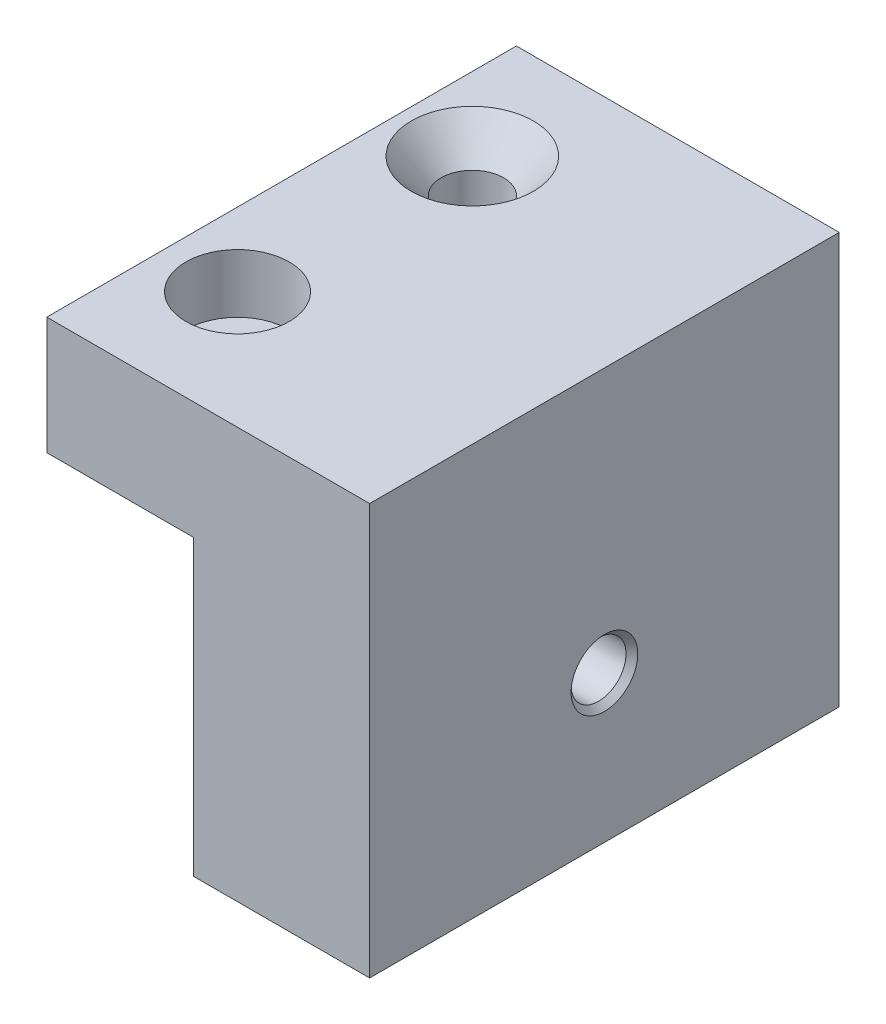
SolidWorks part; units mm, degrees
material "Plain Carbon Steel"
ref_plane "Front Plane" through (0, 0, 0) normal (0, 0, 1) x (1, 0, 0)
ref_plane "Top Plane" through (0, 0, 0) normal (0, 1, 0) x (1, 0, 0)
ref_plane "Right Plane" through (0, 0, 0) normal (1, 0, 0) x (0, 0, -1)
sketch "Block Profile Sketch" plane through (0, 0, 0) normal (0, 0, 1) x (1, 0, 0)
  line L2 (0, 12.7) -> (19.05, 12.7)
  line L3 (0, 0) -> (0, -31.75)
  line L4 (0, -31.75) -> (19.05, -31.75)
  line L5 (19.05, 12.7) -> (19.05, -31.75)
  line L6 (0, 0) -> (-15.875, 0)
  line L8 (0, 12.7) -> (-15.875, 12.7)
  line L9 (-15.875, 0) -> (-15.875, 12.7)
  dimension "D1" = 19.05
  dimension "D2" = 31.75
  dimension "D3" = 44.45
  dimension "D4" = 34.925
extrude "Block Body 2in" add sketch "Block Profile Sketch" along normal blind 50.8
hole_wizard "Side Through Hole Ø0.234" positions "3DSketch1" profile "Sketch3" hole size "A" standard "ANSI Inch" end condition through all
sketch3d "3DSketch1"
  line L0 (0, 0, 50.8) -> (0, 0, 0) construction
  line L1 (0, 0, 0) -> (0, -31.75, 0) construction
  point P1 (0, -15.875, 25.4)
  dimension "D1" = 15.875
  dimension "D2" = 25.4
sketch "Sketch3" plane through (0, -15.875, 25.4) normal (0, 1, 0) x (0, 0, 1)
  line L0 (0, 0) -> (0, 19.05)
  line L1 (0, 19.05) -> (2.9718, 19.05)
  line L2 (2.9718, 19.05) -> (2.9718, 0)
  line L5 (2.9718, 0) -> (0, 0)
  line L11 (0, -6.35) -> (0, 107.95) construction
  dimension "Thru Hole Dia." = 5.9436
  dimension "Thru Hole Depth" = 19.05
chamfer "Side Hole Edge Chamfer" distance 0.635 angle 45 2 edges at (19.05, -15.875, 28.3718) (0, -15.875, 28.3718)
hole_wizard "Dowel Hole Ø0.126" positions "3DSketch2" profile "Sketch4" hole size "1/16" standard "ANSI Inch"
sketch3d "3DSketch2"
  line L0 (-15.875, 0, 0) -> (0, 0, 0) construction
  line L1 (-15.875, 0, 50.8) -> (-15.875, 0, 0) construction
  point P0 (-7.9375, 0, 25.4)
  dimension "D1" = 25.4
  dimension "D2" = 7.9375
sketch "Sketch4" plane through (-7.9375, 0, 25.4) normal (1, 0, 0) x (0, 0, -1)
  line L0 (0, 0) -> (0, 7.62)
  line L1 (0, 7.62) -> (1.6002, 6.0198)
  line L2 (1.6002, 6.0198) -> (1.6002, 0)
  line L5 (1.6002, 0) -> (0, 0)
  line L10 (0, 7.62) -> (-1.6002, 6.0198) construction
  line L11 (0, -6.35) -> (0, 107.95) construction
  dimension "Hole Dia." = 3.2004
  dimension "Hole Depth" = 7.62
  dimension "Drill Angle" = 90
hole_wizard "Countersunk Screw Hole No0" positions "3DSketch3" profile "Sketch5" countersink size "#0" standard "ANSI Inch" end condition through all
sketch3d "3DSketch3"
  line L0 (-15.875, 12.7, 50.8) -> (-15.875, 12.7, 0) construction
  line L1 (19.05, 12.7, 25.4) -> (-15.875, 12.7, 25.4) construction
  line L2 (19.05, 12.7, 50.8) -> (19.05, 12.7, 0) construction
  point P0 (-7.9375, 12.7, 12.7)
  dimension "D1" = 7.9375
  dimension "D2" = 12.7
sketch "Sketch5" plane through (-7.9375, 12.7, 12.7) normal (1, 0, 0) x (0, 0, 1)
  line L0 (0, 0) -> (0, 44.45)
  line L1 (0, 44.45) -> (3.3782, 44.45)
  line L2 (3.3782, 44.45) -> (3.3782, 3.7109)
  line L3 (3.3782, 3.7109) -> (6.604, 0)
  line L5 (6.604, 0) -> (0, 0)
  line L6 (-3.3782, 3.7109) -> (-6.604, 0) construction
  line L11 (0, -6.35) -> (0, 107.95) construction
  dimension "Thru Hole Dia." = 6.7564
  dimension "Thru Hole Depth" = 44.45
  dimension "Near C'Sink Dia." = 13.208
  dimension "Near C'Sink Angle" = 82
hole_wizard "Counterbored Bolt Hole 0.25in" positions "3DSketch4" profile "Sketch6" counterbore size "1/4" standard "ANSI Inch" end condition through all
sketch3d "3DSketch4"
  line L0 (-15.875, 12.7, 50.8) -> (-15.875, 12.7, 0) construction
  line L1 (19.05, 12.7, 25.4) -> (-15.875, 12.7, 25.4) construction
  line L2 (19.05, 12.7, 50.8) -> (19.05, 12.7, 0) construction
  point P0 (-7.9375, 12.7, 38.1)
  dimension "D1" = 7.9375
  dimension "D2" = 12.7
sketch "Sketch6" plane through (-7.9375, 12.7, 38.1) normal (1, 0, 0) x (0, 0, 1)
  line L0 (0, 0) -> (0, 44.45)
  line L1 (0, 44.45) -> (3.3782, 44.45)
  line L3 (3.3782, 44.45) -> (3.3782, 6.35)
  line L4 (3.3782, 6.35) -> (5.588, 6.35)
  line L5 (5.588, 6.35) -> (5.588, 0)
  line L7 (5.588, 0) -> (0, 0)
  line L11 (0, -6.35) -> (0, 107.95) construction
  dimension "Thru Hole Dia." = 6.7564
  dimension "Thru Hole Depth" = 44.45
  dimension "C'Bore Dia." = 11.176
  dimension "C'Bore Depth" = 6.35
sketch "Sketch7" plane through (0, 12.7, 0) normal (0, 1, 0) x (1, 0, 0)
  line L0 (-15.875, -25.4) -> (19.05, -25.4) construction
  line L1 (-15.875, -50.8) -> (-15.875, 0) construction
  line L2 (19.05, -50.8) -> (19.05, 0) construction
